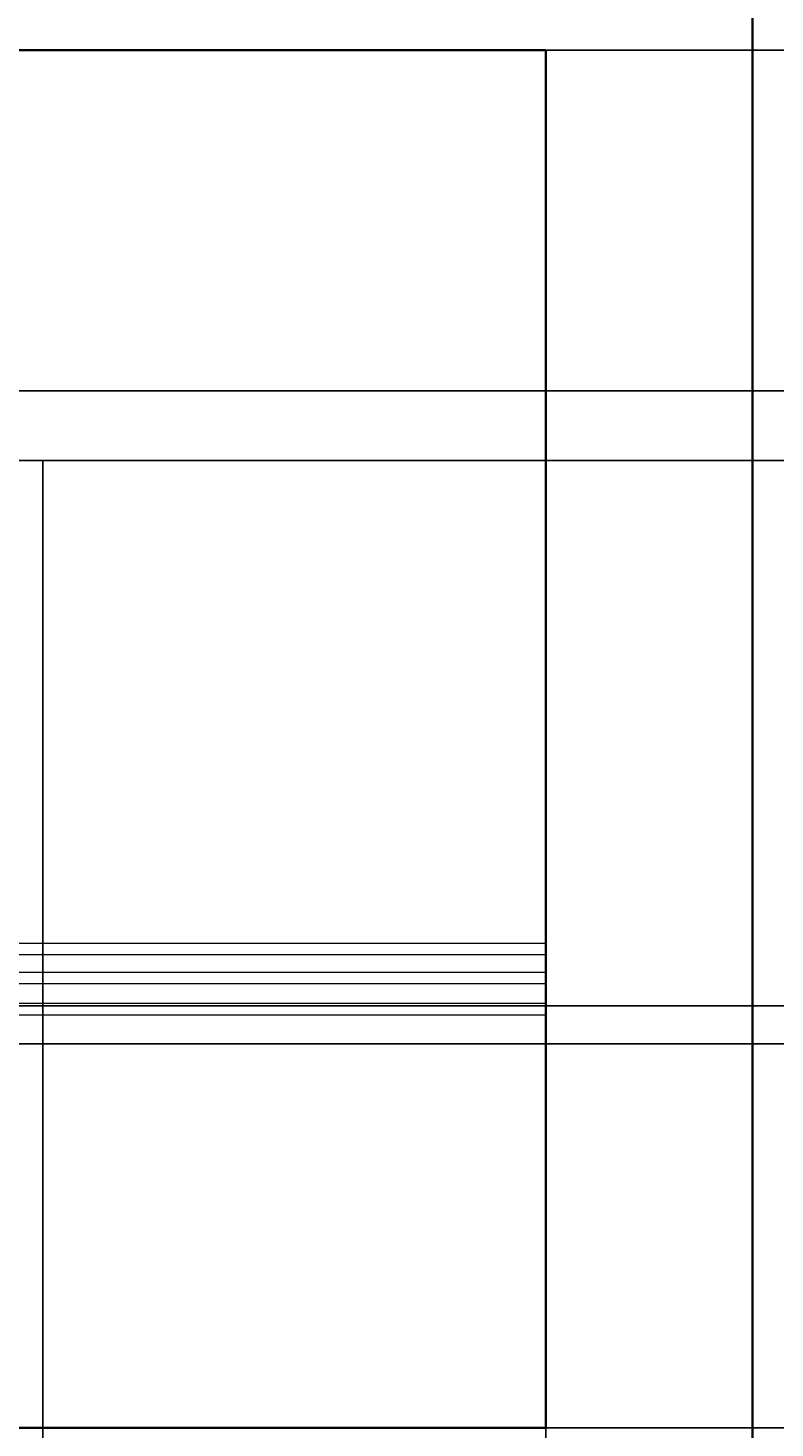
# Model space of a CAD drawing. Units: inches. Extents: x -13 to 809, y 112 to 656.
# Tile 17 of 55: x 274 to 339, y 325 to 446. Entities that reach past the tile are written whole.
import ezdxf

# ---------------------------------------------------------------- set-up
doc = ezdxf.new("R2010")
doc.units = ezdxf.units.IN
doc.header["$MEASUREMENT"] = 0
for name, color, linetype, lineweight in [('A-ANNO-DIMS', 2, 'Continuous', 18), ('A-ELEV', 7, 'Continuous', 35), ('A-ELEV-PATT', 8, 'Continuous', 13), ('A-GLAZ', 4, 'Continuous', 25)]:
    doc.layers.add(name, color=color, linetype=linetype, lineweight=lineweight)
doc.styles.get("Standard").update_dxf_attribs({"font": 'arial.ttf'})
doc.dimstyles.get("Standard").update_dxf_attribs({"dimtxt": 0.625, "dimasz": 0.18, "dimexe": 0.18, "dimexo": 0.0625, "dimgap": 0.09, "dimtad": 0, "dimtih": 1, "dimtoh": 1, "dimdec": 4, "dimzin": 0, "dimdsep": 46, "dimlunit": 4, "dimtxsty": 'Standard', "dimcen": 0.09, "dimadec": 0, "dimazin": 0, "dimtfac": 1, "dimtdec": 4, "dimtofl": 0, "dimtmove": 0, "dimatfit": 3, "dimfxl": 1, "dimtolj": 1, "dimtzin": 0, "dimarcsym": 0})

# ---------------------------------------------------------------- blocks, each defined once
blk = doc.blocks.new('*D39')
at = {"layer": 'A-ANNO-DIMS', "color": 0, "lineweight": -2, "transparency": 16777216}
for p, q in [((341.34, 524.28), (-12.1, 524.28)), ((-11.92, 524.1), (-11.92, 406.78)), ((-11.92, 288.63), (-11.92, 405.96)), ((341.34, 288.45), (-12.1, 288.45))]:
    blk.add_line(p, q, dxfattribs=at)
at = {"layer": 'A-ANNO-DIMS', "color": 0, "transparency": 16777216}
for points in [[(-11.95, 524.1), (-11.89, 524.1), (-11.92, 524.28)], [(-11.95, 288.63), (-11.89, 288.63), (-11.92, 288.45)]]:
    blk.add_solid(points, dxfattribs=at)
at = {"layer": 'Defpoints', "color": 0, "transparency": 16777216}
for p in [(-11.92, 524.28), (341.41, 524.28), (341.41, 288.45)]:
    blk.add_point(p, dxfattribs=at)
at = {"layer": 'A-ANNO-DIMS', "color": 0, "transparency": 16777216, "insert": (-11.92, 406.37), "char_height": 0.625, "attachment_point": 5}
blk.add_mtext('\\A1;235.83', dxfattribs=at)
blk = doc.blocks.new('*D41')
at = {"layer": 'A-ANNO-DIMS', "color": 0, "lineweight": -2, "transparency": 16777216}
for p, q in [((471.04, 357.98), (-12.1, 357.98)), ((-11.92, 357.8), (-11.92, 335.98)), ((-11.92, 313.35), (-11.92, 335.16)), ((471.04, 313.17), (-12.1, 313.17))]:
    blk.add_line(p, q, dxfattribs=at)
at = {"layer": 'A-ANNO-DIMS', "color": 0, "transparency": 16777216}
for points in [[(-11.95, 357.8), (-11.89, 357.8), (-11.92, 357.98)], [(-11.95, 313.35), (-11.89, 313.35), (-11.92, 313.17)]]:
    blk.add_solid(points, dxfattribs=at)
at = {"layer": 'Defpoints', "color": 0, "transparency": 16777216}
for p in [(-11.92, 357.98), (471.1, 357.98), (471.1, 313.17)]:
    blk.add_point(p, dxfattribs=at)
at = {"layer": 'A-ANNO-DIMS', "color": 0, "transparency": 16777216, "insert": (-11.92, 335.57), "char_height": 0.625, "attachment_point": 5}
blk.add_mtext('\\A1;44.81', dxfattribs=at)
blk = doc.blocks.new('*D42')
at = {"layer": 'A-ANNO-DIMS', "color": 0, "lineweight": -2, "transparency": 16777216}
for p, q in [((471.04, 414.86), (-12.1, 414.86)), ((-11.92, 414.68), (-11.92, 386.83)), ((-11.92, 358.16), (-11.92, 386.01)), ((471.04, 357.98), (-12.1, 357.98))]:
    blk.add_line(p, q, dxfattribs=at)
at = {"layer": 'A-ANNO-DIMS', "color": 0, "transparency": 16777216}
for points in [[(-11.95, 414.68), (-11.89, 414.68), (-11.92, 414.86)], [(-11.95, 358.16), (-11.89, 358.16), (-11.92, 357.98)]]:
    blk.add_solid(points, dxfattribs=at)
at = {"layer": 'Defpoints', "color": 0, "transparency": 16777216}
for p in [(-11.92, 414.86), (471.1, 414.86), (471.1, 357.98)]:
    blk.add_point(p, dxfattribs=at)
at = {"layer": 'A-ANNO-DIMS', "color": 0, "transparency": 16777216, "insert": (-11.92, 386.42), "char_height": 0.625, "attachment_point": 5}
blk.add_mtext('\\A1;56.88', dxfattribs=at)
blk = doc.blocks.new('*D43')
at = {"layer": 'A-ANNO-DIMS', "color": 0, "lineweight": -2, "transparency": 16777216}
for p, q in [((471.04, 470.88), (-12.1, 470.88)), ((-11.92, 470.7), (-11.92, 443.28)), ((-11.92, 415.04), (-11.92, 442.46)), ((471.04, 414.86), (-12.1, 414.86))]:
    blk.add_line(p, q, dxfattribs=at)
at = {"layer": 'A-ANNO-DIMS', "color": 0, "transparency": 16777216}
for points in [[(-11.95, 470.7), (-11.89, 470.7), (-11.92, 470.88)], [(-11.95, 415.04), (-11.89, 415.04), (-11.92, 414.86)]]:
    blk.add_solid(points, dxfattribs=at)
at = {"layer": 'Defpoints', "color": 0, "transparency": 16777216}
for p in [(-11.92, 470.88), (471.1, 470.88), (471.1, 414.86)]:
    blk.add_point(p, dxfattribs=at)
at = {"layer": 'A-ANNO-DIMS', "color": 0, "transparency": 16777216, "insert": (-11.92, 442.87), "char_height": 0.625, "attachment_point": 5}
blk.add_mtext('\\A1;56.02', dxfattribs=at)
blk = doc.blocks.new('*D46')
at = {"layer": 'A-ANNO-DIMS', "color": 0, "lineweight": -2, "transparency": 16777216}
for p, q in [((160.98, 408.79), (807.77, 408.79)), ((807.59, 408.61), (807.59, 367.07)), ((807.59, 324.7), (807.59, 366.25)), ((160.98, 324.52), (807.77, 324.52))]:
    blk.add_line(p, q, dxfattribs=at)
at = {"layer": 'A-ANNO-DIMS', "color": 0, "transparency": 16777216}
for points in [[(807.56, 408.61), (807.62, 408.61), (807.59, 408.79)], [(807.56, 324.7), (807.62, 324.7), (807.59, 324.52)]]:
    blk.add_solid(points, dxfattribs=at)
at = {"layer": 'Defpoints', "color": 0, "transparency": 16777216}
for p in [(160.92, 408.79), (807.59, 408.79), (160.92, 324.52)]:
    blk.add_point(p, dxfattribs=at)
at = {"layer": 'A-ANNO-DIMS', "color": 0, "transparency": 16777216, "insert": (807.59, 366.66), "char_height": 0.625, "attachment_point": 5}
blk.add_mtext('\\A1;84.27', dxfattribs=at)
blk = doc.blocks.new('*D47')
at = {"layer": 'A-ANNO-DIMS', "color": 0, "lineweight": -2, "transparency": 16777216}
for p, q in [((275.78, 408.79), (807.77, 408.79)), ((807.59, 408.61), (807.59, 385.45)), ((807.59, 361.47), (807.59, 384.63)), ((275.78, 361.29), (807.77, 361.29))]:
    blk.add_line(p, q, dxfattribs=at)
at = {"layer": 'A-ANNO-DIMS', "color": 0, "transparency": 16777216}
for points in [[(807.56, 408.61), (807.62, 408.61), (807.59, 408.79)], [(807.56, 361.47), (807.62, 361.47), (807.59, 361.29)]]:
    blk.add_solid(points, dxfattribs=at)
at = {"layer": 'Defpoints', "color": 0, "transparency": 16777216}
for p in [(275.71, 408.79), (807.59, 408.79), (275.71, 361.29)]:
    blk.add_point(p, dxfattribs=at)
at = {"layer": 'A-ANNO-DIMS', "color": 0, "transparency": 16777216, "insert": (807.59, 385.04), "char_height": 0.625, "attachment_point": 5}
blk.add_mtext('\\A1;47.5', dxfattribs=at)
blk = doc.blocks.new('*D48')
at = {"layer": 'A-ANNO-DIMS', "color": 0, "lineweight": -2, "transparency": 16777216}
for p, q in [((319.57, 444.52), (807.77, 444.52)), ((807.59, 444.34), (807.59, 384.93)), ((807.59, 324.7), (807.59, 384.11)), ((319.57, 324.52), (807.77, 324.52))]:
    blk.add_line(p, q, dxfattribs=at)
at = {"layer": 'A-ANNO-DIMS', "color": 0, "transparency": 16777216}
for points in [[(807.56, 444.34), (807.62, 444.34), (807.59, 444.52)], [(807.56, 324.7), (807.62, 324.7), (807.59, 324.52)]]:
    blk.add_solid(points, dxfattribs=at)
at = {"layer": 'Defpoints', "color": 0, "transparency": 16777216}
for p in [(319.51, 444.52), (807.59, 444.52), (319.51, 324.52)]:
    blk.add_point(p, dxfattribs=at)
at = {"layer": 'A-ANNO-DIMS', "color": 0, "transparency": 16777216, "insert": (807.59, 384.52), "char_height": 0.625, "attachment_point": 5}
blk.add_mtext('\\A1;120', dxfattribs=at)
blk = doc.blocks.new('*D105')
at = {"layer": 'A-ANNO-DIMS', "color": 0, "lineweight": -2, "transparency": 16777216}
for p, q in [((319.76, 452.56), (807.77, 452.56)), ((807.59, 452.38), (807.59, 448.95)), ((807.59, 444.7), (807.59, 448.13)), ((319.57, 444.52), (807.77, 444.52))]:
    blk.add_line(p, q, dxfattribs=at)
at = {"layer": 'A-ANNO-DIMS', "color": 0, "transparency": 16777216}
for points in [[(807.56, 452.38), (807.62, 452.38), (807.59, 452.56)], [(807.56, 444.7), (807.62, 444.7), (807.59, 444.52)]]:
    blk.add_solid(points, dxfattribs=at)
at = {"layer": 'Defpoints', "color": 0, "transparency": 16777216}
for p in [(319.7, 452.56), (319.51, 444.52), (807.59, 444.52)]:
    blk.add_point(p, dxfattribs=at)
at = {"layer": 'A-ANNO-DIMS', "color": 0, "transparency": 16777216, "insert": (807.59, 448.54), "char_height": 0.625, "attachment_point": 5}
blk.add_mtext('\\A1;8.043', dxfattribs=at)
blk = doc.blocks.new('*D112')
at = {"layer": 'A-ANNO-DIMS', "color": 0, "lineweight": -2, "transparency": 16777216}
for p, q in [((210.08, 361.23), (210.08, 112.34)), ((275.71, 361.23), (275.71, 112.34)), ((210.26, 112.52), (241.75, 112.52)), ((275.53, 112.52), (244.04, 112.52))]:
    blk.add_line(p, q, dxfattribs=at)
at = {"layer": 'A-ANNO-DIMS', "color": 0, "transparency": 16777216}
for points in [[(210.26, 112.55), (210.26, 112.49), (210.08, 112.52)], [(275.53, 112.55), (275.53, 112.49), (275.71, 112.52)]]:
    blk.add_solid(points, dxfattribs=at)
at = {"layer": 'Defpoints', "color": 0, "transparency": 16777216}
for p in [(210.08, 361.29), (275.71, 361.29), (275.71, 112.52)]:
    blk.add_point(p, dxfattribs=at)
at = {"layer": 'A-ANNO-DIMS', "color": 0, "transparency": 16777216, "insert": (242.9, 112.52), "char_height": 0.625, "attachment_point": 5}
blk.add_mtext('\\A1;65.64', dxfattribs=at)
blk = doc.blocks.new('*D113')
at = {"layer": 'A-ANNO-DIMS', "color": 0, "lineweight": -2, "transparency": 16777216}
for p, q in [((275.71, 361.23), (275.71, 112.34)), ((319.51, 324.46), (319.51, 112.34)), ((275.89, 112.52), (296.45, 112.52)), ((319.33, 112.52), (298.77, 112.52))]:
    blk.add_line(p, q, dxfattribs=at)
at = {"layer": 'A-ANNO-DIMS', "color": 0, "transparency": 16777216}
for points in [[(275.89, 112.55), (275.89, 112.49), (275.71, 112.52)], [(319.33, 112.55), (319.33, 112.49), (319.51, 112.52)]]:
    blk.add_solid(points, dxfattribs=at)
at = {"layer": 'Defpoints', "color": 0, "transparency": 16777216}
for p in [(275.71, 361.29), (319.51, 324.52), (319.51, 112.52)]:
    blk.add_point(p, dxfattribs=at)
at = {"layer": 'A-ANNO-DIMS', "color": 0, "transparency": 16777216, "insert": (297.61, 112.52), "char_height": 0.625, "attachment_point": 5}
blk.add_mtext('\\A1;43.79', dxfattribs=at)

msp = doc.modelspace()

# ---------------------------------------------------------------- linework, layer by layer
at = {"layer": 'A-ELEV'}
for p, q in [((337.5074, 462.5199), (337.5074, 306.5199)), ((113.0469, 444.5199), (319.5074, 444.5199)), ((319.5074, 444.5199), (319.5074, 324.5199)), ((113.0469, 324.5199), (319.5074, 324.5199))]:
    msp.add_line(p, q, dxfattribs=at)
at = {"layer": 'A-ELEV-PATT'}
for p, q in [((113.0469, 366.753), (319.5074, 366.753)), ((113.0469, 365.753), (319.5074, 365.753)), ((113.0469, 364.2343), (319.5074, 364.2343)), ((113.0469, 363.2343), (319.5074, 363.2343)), ((113.0469, 361.5199), (319.5074, 361.5199)), ((113.0469, 360.5199), (319.5074, 360.5199))]:
    msp.add_line(p, q, dxfattribs=at)
at = {"layer": 'A-GLAZ'}
msp.add_lwpolyline([(210.0791, 408.7939), (275.7145, 408.7939), (275.7145, 361.2915), (210.0791, 361.2915)], close=True, dxfattribs=at)

# ---------------------------------------------------------------- dimensions: what is measured, and where the dimension line sits
at = {"layer": 'A-ANNO-DIMS'}
for base, p1, p2, override, picture, middle in [((-11.9191, 524.281), (341.4072, 288.4508), (341.4072, 524.281), {"dimdec": 2, "dimlfac": 1, "dimrnd": 0, "dimzin": 0, "dimdsep": 46, "dimlunit": 2}, '*D39', (-11.9191, 406.3659)), ((-11.9191, 470.8765), (471.0998, 414.8594), (471.0998, 470.8765), {"dimdec": 2, "dimlfac": 1, "dimrnd": 0, "dimzin": 0, "dimdsep": 46, "dimlunit": 2}, '*D43', (-11.9191, 442.8679)), ((807.5888, 444.5199), (319.7004, 452.5629), (319.5074, 444.5199), {"dimdec": 3, "dimlfac": 1, "dimrnd": 0, "dimzin": 0, "dimdsep": 46, "dimlunit": 2}, '*D105', (807.5888, 448.5414)), ((807.5888, 444.5199), (319.5074, 324.5199), (319.5074, 444.5199), {"dimdec": 0, "dimlfac": 1, "dimrnd": 0, "dimzin": 0, "dimdsep": 46, "dimlunit": 2}, '*D48', (807.5888, 384.5199)), ((-11.9191, 414.8594), (471.0998, 357.9804), (471.0998, 414.8594), {"dimdec": 2, "dimlfac": 1, "dimrnd": 0, "dimzin": 0, "dimdsep": 46, "dimlunit": 2}, '*D42', (-11.9191, 386.4199)), ((807.5888, 408.7939), (160.9184, 324.5199), (160.9184, 408.7939), {"dimdec": 2, "dimlfac": 1, "dimrnd": 0, "dimzin": 0, "dimdsep": 46, "dimlunit": 2}, '*D46', (807.5888, 366.6569)), ((807.5888, 408.7939), (275.7145, 361.2915), (275.7145, 408.7939), {"dimdec": 1, "dimlfac": 1, "dimrnd": 0, "dimzin": 0, "dimdsep": 46, "dimlunit": 2}, '*D47', (807.5888, 385.0427)), ((-11.9191, 357.9804), (471.0998, 313.1667), (471.0998, 357.9804), {"dimdec": 2, "dimlfac": 1, "dimrnd": 0, "dimzin": 0, "dimdsep": 46, "dimlunit": 2}, '*D41', (-11.9191, 335.5735))]:
    dim = msp.add_linear_dim(base=base, p1=p1, p2=p2, angle=90, dimstyle='Standard', override=override, dxfattribs=at)
    dim.commit()
    dim.dimension.update_dxf_attribs({"geometry": picture, "text_midpoint": middle})
for base, p1, p2, picture, middle in [((275.7145, 112.5199), (210.0791, 361.2915), (275.7145, 361.2915), '*D112', (242.8968, 112.5199)), ((319.5074, 112.5199), (275.7145, 361.2915), (319.5074, 324.5199), '*D113', (297.611, 112.5199))]:
    dim = msp.add_linear_dim(base=base, p1=p1, p2=p2, dimstyle='Standard', override={"dimdec": 2, "dimlfac": 1, "dimrnd": 0, "dimzin": 0, "dimdsep": 46, "dimlunit": 2}, dxfattribs=at)
    dim.commit()
    dim.dimension.update_dxf_attribs({"geometry": picture, "text_midpoint": middle})

doc.saveas('drawing.dxf')
